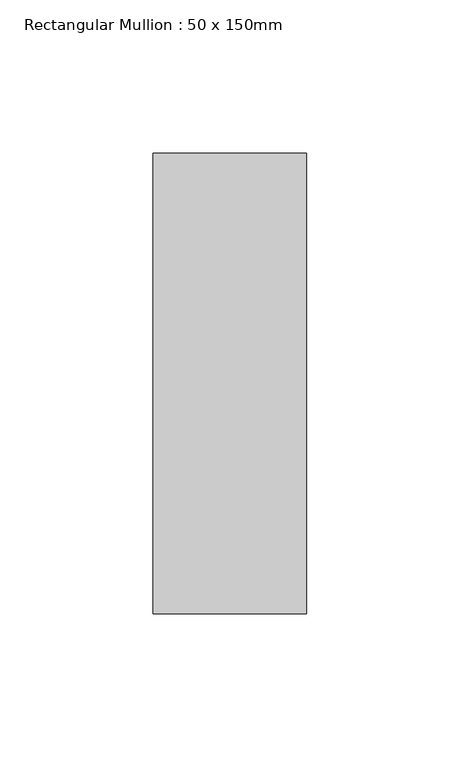
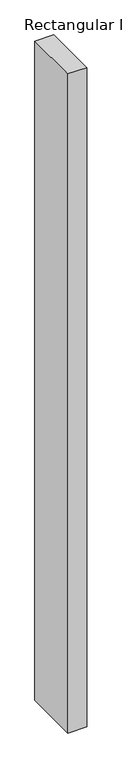
"""IFC4 building model written with IfcOpenShell, lengths in millimetres: member geometry, Rectangular Mullion : 50 x 150mm."""

from ifc_helpers import new_model, si_unit, frame, origin, place, context, project, spatial, polyline, outline, extrude, source, transform, mapped, element, save


def rectangular_mullion_50_x_150mm_aaee7d48(model_context):
    return source(origin(), model_context, "Body", "SweptSolid", [
        extrude(outline(polyline([(0.0, 75.0), (0.0, -75.0), (-50.0, -75.0), (-50.0, 75.0), (0.0, 75.0)])), frame((0.0, 0.0, -1830.0), z_axis=(0.0, 0.0, 1.0), x_axis=(1.0, 0.0, 0.0)), (0.0, 0.0, 1.0), 1830.0),
    ])


if __name__ == "__main__":
    model = new_model("IFC4")
    model_context = context("Model", 3, world=origin())
    ifc_project = project(units=[si_unit("LENGTHUNIT", "METRE", prefix="MILLI")], contexts=[model_context])
    site = spatial("IfcSite", under=ifc_project)
    building = spatial("IfcBuilding", under=site)
    placement = place(None, origin())
    rectangular_mullion_50_x_150mm_shape = rectangular_mullion_50_x_150mm_aaee7d48(model_context)
    element("IfcMember", 1, ObjectType="Rectangular Mullion : 50 x 150mm", at=placement, inside=building, context=model_context, shape_type="MappedRepresentation", body=[
        mapped(rectangular_mullion_50_x_150mm_shape, transform((0.0, 0.0, 0.0), x_axis=(1.0, 0.0, 0.0), y_axis=(0.0, 1.0, 0.0), z_axis=(0.0, 0.0, 1.0))),
    ])
    save(model, "model.ifc")

# Revit data of these elements
# Type "Rectangular Mullion : 50 x 150mm"
#   built-in parameter 1007304 = 0.492126 (stored number, unit not read)
#   built-in parameter 1007301 = 0.082021 (stored number, unit not read)
#   built-in parameter 1007300 = 0.082021 (stored number, unit not read)
# Element 1 (IfcMember, "Rectangular Mullion : 50 x 150mm")
#   Materials on its faces: "Aluminium"
# Materials
#   "Aluminium": class "Metal", colour RGB 247 247 247, transparency 0, Description = "Aluminium 6061", Cost = 0
